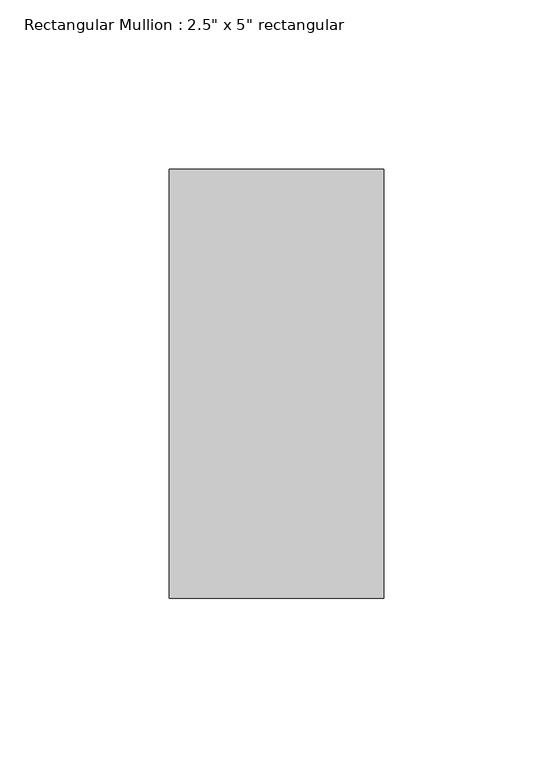
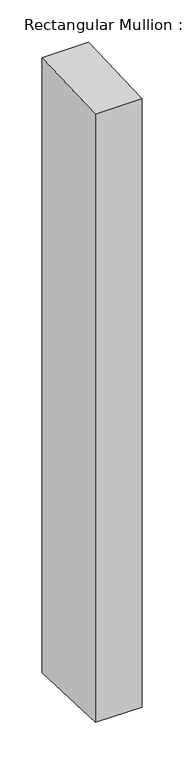
"""IFC4 building model written with IfcOpenShell, lengths in millimetres: member geometry."""

from ifc_helpers import new_model, si_unit, frame, origin, place, context, project, spatial, polyline, outline, extrude, source, transform, mapped, element, save


def member_3197f2db(model_context):
    return source(origin(), model_context, "Body", "SweptSolid", [
        extrude(outline(polyline([(-63.5, -2.5814971), (63.5, 2.5814971), (63.5, -887.1160389), (-63.5, -882.3171123), (-63.5, -2.5814971)])), frame((-63.5, 0.0, 0.0), z_axis=(1.0, 0.0, 0.0), x_axis=(0.0, 1.0, 0.0)), (0.0, 0.0, 1.0), 63.5),
    ])


if __name__ == "__main__":
    model = new_model("IFC4")
    model_context = context("Model", 3, world=origin())
    ifc_project = project(units=[si_unit("LENGTHUNIT", "METRE", prefix="MILLI")], contexts=[model_context])
    site = spatial("IfcSite", under=ifc_project)
    building = spatial("IfcBuilding", under=site)
    placement = place(None, origin())
    member_shape = member_3197f2db(model_context)
    element("IfcMember", 1, ObjectType="Rectangular Mullion : 2.5\" x 5\" rectangular", at=placement, inside=building, context=model_context, shape_type="MappedRepresentation", body=[
        mapped(member_shape, transform((0.0, 0.0, 0.0), x_axis=(1.0, 0.0, 0.0), y_axis=(0.0, 1.0, 0.0), z_axis=(0.0, 0.0, 1.0))),
    ])
    save(model, "model.ifc")

# Revit data of these elements
# Type "Rectangular Mullion : 2.5\" x 5\" rectangular"
#   built-in parameter 1007304 = 0.416667 (stored number, unit not read)
#   built-in parameter 1007301 = 0.104167 (stored number, unit not read)
#   built-in parameter 1007300 = 0.104167 (stored number, unit not read)
# Element 1 (IfcMember, "Rectangular Mullion : 2.5\" x 5\" rectangular")
#   Materials on its faces: "Aluminum"
# Materials
#   "Aluminum": class "Metal", colour RGB 247 247 247, transparency 0, Description = "Aluminum 6061", Cost = 0
